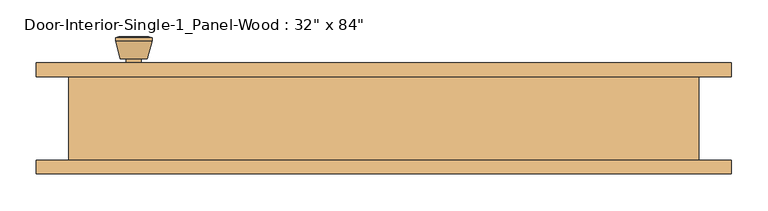
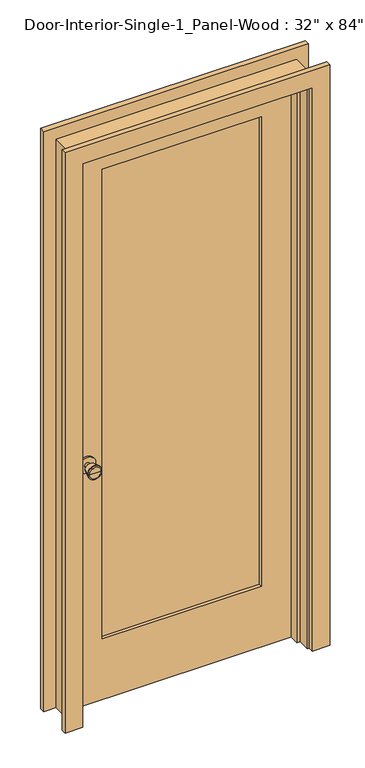
"""IFC4 building model written with IfcOpenShell, lengths in millimetres: door geometry."""

from ifc_helpers import new_model, si_unit, point, frame, frame_2d, origin, place, context, project, spatial, polyline, circle_curve, trimmed, segment, composite_curve, outline, extrude, faceted_brep, source, transform, mapped, element, save
from ifc_brep_helpers import plane_surface, cylinder_surface, revolved_surface, advanced_brep


def door_643e272e(model_context):
    return source(origin(), model_context, "Body", "SolidModel", [
        advanced_brep(
        [(-342.9, 13.05, 914.4), (-332.9, 13.05, 914.4), (-352.9, 13.05, 914.4), (-322.4241324, -35.95, 914.4), (-342.9, -35.95, 914.4), (-363.3758676, -35.95, 914.4), (-317.9, -34.1221319, 914.4), (-367.9, -34.1221319, 914.4), (-317.9, -30.6584537, 914.4), (-367.9, -30.6584537, 914.4), (-324.263764, -5.95, 914.4), (-361.536236, -5.95, 914.4), (-332.9, -5.95, 914.4), (-352.9, -5.95, 914.4)],
        [
            (0, 1),
            (1, 2, circle_curve(frame((-342.9, 13.05, 914.4), z_axis=(0.0, 1.0, 0.0), x_axis=(-1.0, 0.0, 0.0)), 10.0)),
            (2, 0),
            (2, 1, circle_curve(frame((-342.9, 13.05, 914.4), z_axis=(0.0, 1.0, 0.0), x_axis=(-1.0, 0.0, 0.0)), 10.0)),
            (3, 4),
            (4, 5),
            (5, 3, circle_curve(frame((-342.9, -35.95, 914.4), z_axis=(0.0, -1.0, 0.0), x_axis=(-1.0, 0.0, 0.0)), 20.4758676)),
            (3, 5, circle_curve(frame((-342.9, -35.95, 914.4), z_axis=(0.0, -1.0, 0.0), x_axis=(-1.0, 0.0, 0.0)), 20.4758676)),
            (6, 3),
            (5, 7),
            (7, 6, circle_curve(frame((-342.9, -34.1221319, 914.4), z_axis=(0.0, -1.0, 0.0), x_axis=(-1.0, 0.0, 0.0)), 25.0)),
            (6, 7, circle_curve(frame((-342.9, -34.1221319, 914.4), z_axis=(0.0, -1.0, 0.0), x_axis=(-1.0, 0.0, 0.0)), 25.0)),
            (8, 6),
            (7, 9),
            (9, 8, circle_curve(frame((-342.9, -30.6584537, 914.4), z_axis=(0.0, -1.0, 0.0), x_axis=(-1.0, 0.0, 0.0)), 25.0)),
            (8, 9, circle_curve(frame((-342.9, -30.6584537, 914.4), z_axis=(0.0, -1.0, 0.0), x_axis=(-1.0, 0.0, 0.0)), 25.0)),
            (10, 8),
            (9, 11),
            (11, 10, circle_curve(frame((-342.9, -5.95, 914.4), z_axis=(0.0, -1.0, 0.0), x_axis=(-1.0, 0.0, 0.0)), 18.636236)),
            (10, 11, circle_curve(frame((-342.9, -5.95, 914.4), z_axis=(0.0, -1.0, 0.0), x_axis=(-1.0, 0.0, 0.0)), 18.636236)),
            (12, 10),
            (11, 13),
            (13, 12, circle_curve(frame((-342.9, -5.95, 914.4), z_axis=(0.0, -1.0, 0.0), x_axis=(-1.0, 0.0, 0.0)), 10.0)),
            (12, 13, circle_curve(frame((-342.9, -5.95, 914.4), z_axis=(0.0, -1.0, 0.0), x_axis=(-1.0, 0.0, 0.0)), 10.0)),
            (1, 12),
            (13, 2),
        ],
        [
            plane_surface(frame((-342.9, 13.05, 914.4), z_axis=(0.0, 1.0, 0.0), x_axis=(-1.0, 0.0, 0.0))),
            plane_surface(frame((-342.9, -35.95, 914.4), z_axis=(0.0, -1.0, 0.0), x_axis=(-1.0, 0.0, 0.0))),
            revolved_surface(polyline([(-363.3758676, -35.95, 914.4), (-367.9, -34.1221319, 914.4)]), (-342.9, 13.05, 914.4), (0.0, 1.0, 0.0)),
            cylinder_surface(frame((-342.9, 13.05, 914.4), z_axis=(0.0, 1.0, 0.0), x_axis=(-1.0, 0.0, 0.0)), 25.0),
            revolved_surface(polyline([(-367.9, -30.6584537, 914.4), (-361.536236, -5.95, 914.4)]), (-342.9, 13.05, 914.4), (0.0, 1.0, 0.0)),
            plane_surface(frame((-342.9, -5.95, 914.4), z_axis=(0.0, 1.0, 0.0), x_axis=(-1.0, 0.0, 0.0))),
            cylinder_surface(frame((-342.9, 13.05, 914.4), z_axis=(0.0, 1.0, 0.0), x_axis=(-1.0, 0.0, 0.0)), 10.0),
        ],
        [
            (0, [[1, 2, 3]]),
            (0, [[-3, 4, -1]]),
            (1, [[5, 6, 7]]),
            (1, [[-6, -5, 8]]),
            (2, [[9, -7, 10, 11]]),
            (2, [[-10, -8, -9, 12]]),
            (3, [[13, -11, 14, 15]]),
            (3, [[-14, -12, -13, 16]]),
            (4, [[17, -15, 18, 19]]),
            (4, [[-18, -16, -17, 20]]),
            (5, [[21, -19, 22, 23]]),
            (5, [[-22, -20, -21, 24]]),
            (6, [[25, -23, 26, -2]]),
            (6, [[-26, -24, -25, -4]]),
        ],
    ),
        extrude(outline(composite_curve([segment(trimmed(circle_curve(frame_2d((914.4, -342.9)), 30.0), [point((914.4, -372.9))], [point((914.4, -312.9))], False, "CARTESIAN"), True, "CONTINUOUS"), segment(trimmed(circle_curve(frame_2d((914.4, -342.9)), 30.0), [point((914.4, -312.9))], [point((914.4, -372.9))], False, "CARTESIAN"), True, "CONTINUOUS")], self_intersect=False)), frame((0.0, 13.05, 0.0), z_axis=(0.0, 1.0, 0.0), x_axis=(0.0, 0.0, 1.0)), (0.0, 0.0, 1.0), 6.0),
        advanced_brep(
        [(-342.9, 59.975, 914.4), (-352.9, 59.975, 914.4), (-332.9, 59.975, 914.4), (-322.4241324, 108.975, 914.4), (-363.3758676, 108.975, 914.4), (-342.9, 108.975, 914.4), (-317.9, 107.1471319, 914.4), (-367.9, 107.1471319, 914.4), (-317.9, 103.6834537, 914.4), (-367.9, 103.6834537, 914.4), (-324.263764, 78.975, 914.4), (-361.536236, 78.975, 914.4), (-332.9, 78.975, 914.4), (-352.9, 78.975, 914.4)],
        [
            (0, 1),
            (1, 2, circle_curve(frame((-342.9, 59.975, 914.4), z_axis=(0.0, -1.0, 0.0), x_axis=(-1.0, 0.0, 0.0)), 10.0)),
            (2, 0),
            (2, 1, circle_curve(frame((-342.9, 59.975, 914.4), z_axis=(0.0, -1.0, 0.0), x_axis=(-1.0, 0.0, 0.0)), 10.0)),
            (3, 4, circle_curve(frame((-342.9, 108.975, 914.4), z_axis=(0.0, 1.0, 0.0), x_axis=(-1.0, 0.0, 0.0)), 20.4758676)),
            (4, 5),
            (5, 3),
            (4, 3, circle_curve(frame((-342.9, 108.975, 914.4), z_axis=(0.0, 1.0, 0.0), x_axis=(-1.0, 0.0, 0.0)), 20.4758676)),
            (6, 7, circle_curve(frame((-342.9, 107.1471319, 914.4), z_axis=(0.0, 1.0, 0.0), x_axis=(-1.0, 0.0, 0.0)), 25.0)),
            (7, 4),
            (3, 6),
            (7, 6, circle_curve(frame((-342.9, 107.1471319, 914.4), z_axis=(0.0, 1.0, 0.0), x_axis=(-1.0, 0.0, 0.0)), 25.0)),
            (8, 9, circle_curve(frame((-342.9, 103.6834537, 914.4), z_axis=(0.0, 1.0, 0.0), x_axis=(-1.0, 0.0, 0.0)), 25.0)),
            (9, 7),
            (6, 8),
            (9, 8, circle_curve(frame((-342.9, 103.6834537, 914.4), z_axis=(0.0, 1.0, 0.0), x_axis=(-1.0, 0.0, 0.0)), 25.0)),
            (10, 11, circle_curve(frame((-342.9, 78.975, 914.4), z_axis=(0.0, 1.0, 0.0), x_axis=(-1.0, 0.0, 0.0)), 18.636236)),
            (11, 9),
            (8, 10),
            (11, 10, circle_curve(frame((-342.9, 78.975, 914.4), z_axis=(0.0, 1.0, 0.0), x_axis=(-1.0, 0.0, 0.0)), 18.636236)),
            (12, 13, circle_curve(frame((-342.9, 78.975, 914.4), z_axis=(0.0, 1.0, 0.0), x_axis=(-1.0, 0.0, 0.0)), 10.0)),
            (13, 11),
            (10, 12),
            (13, 12, circle_curve(frame((-342.9, 78.975, 914.4), z_axis=(0.0, 1.0, 0.0), x_axis=(-1.0, 0.0, 0.0)), 10.0)),
            (1, 13),
            (12, 2),
        ],
        [
            plane_surface(frame((-342.9, 59.975, 914.4), z_axis=(0.0, -1.0, 0.0), x_axis=(-1.0, 0.0, 0.0))),
            plane_surface(frame((-342.9, 108.975, 914.4), z_axis=(0.0, 1.0, 0.0), x_axis=(-1.0, 0.0, 0.0))),
            revolved_surface(polyline([(-363.3758676, 108.975, 914.4), (-367.9, 107.1471319, 914.4)]), (-342.9, 59.975, 914.4), (0.0, -1.0, 0.0)),
            cylinder_surface(frame((-342.9, 59.975, 914.4), z_axis=(0.0, -1.0, 0.0), x_axis=(-1.0, 0.0, 0.0)), 25.0),
            revolved_surface(polyline([(-367.9, 103.6834537, 914.4), (-361.536236, 78.975, 914.4)]), (-342.9, 59.975, 914.4), (0.0, -1.0, 0.0)),
            plane_surface(frame((-342.9, 78.975, 914.4), z_axis=(0.0, -1.0, 0.0), x_axis=(-1.0, 0.0, 0.0))),
            cylinder_surface(frame((-342.9, 59.975, 914.4), z_axis=(0.0, -1.0, 0.0), x_axis=(-1.0, 0.0, 0.0)), 10.0),
        ],
        [
            (0, [[1, 2, 3]]),
            (0, [[-3, 4, -1]]),
            (1, [[5, 6, 7]]),
            (1, [[8, -7, -6]]),
            (2, [[9, 10, -5, 11]]),
            (2, [[12, -11, -8, -10]]),
            (3, [[13, 14, -9, 15]]),
            (3, [[16, -15, -12, -14]]),
            (4, [[17, 18, -13, 19]]),
            (4, [[20, -19, -16, -18]]),
            (5, [[21, 22, -17, 23]]),
            (5, [[24, -23, -20, -22]]),
            (6, [[-2, 25, -21, 26]]),
            (6, [[-4, -26, -24, -25]]),
        ],
    ),
        extrude(outline(composite_curve([segment(trimmed(circle_curve(frame_2d((914.4, -342.9)), 30.0), [point((914.4, -372.9))], [point((914.4, -312.9))], False, "CARTESIAN"), True, "CONTINUOUS"), segment(trimmed(circle_curve(frame_2d((914.4, -342.9)), 30.0), [point((914.4, -312.9))], [point((914.4, -372.9))], False, "CARTESIAN"), True, "CONTINUOUS")], self_intersect=False)), frame((0.0, 53.975, 0.0), z_axis=(0.0, 1.0, 0.0), x_axis=(0.0, 0.0, 1.0)), (0.0, 0.0, 1.0), 6.0),
        faceted_brep([(431.8, 53.975, 0.0), (431.8, -60.325, 0.0), (406.4, -60.325, 0.0), (406.4, -15.875, 0.0), (393.7, -15.875, 0.0), (393.7, 19.05, 0.0), (406.4, 19.05, 0.0), (406.4, 53.975, 0.0), (431.8, 53.975, 2159.0), (431.8, -60.325, 2159.0), (-431.8, -60.325, 2159.0), (-431.8, -60.325, 0.0), (-406.4, -60.325, 0.0), (-406.4, -60.325, 2133.6), (406.4, -60.325, 2133.6), (406.4, -15.875, 2133.6), (-406.4, -15.875, 2133.6), (-406.4, -15.875, 0.0), (-393.7, -15.875, 0.0), (-393.7, -15.875, 2120.9), (393.7, -15.875, 2120.9), (393.7, 19.05, 2120.9), (-393.7, 19.05, 2120.9), (-393.7, 19.05, 0.0), (-406.4, 19.05, 0.0), (-406.4, 19.05, 2133.6), (406.4, 19.05, 2133.6), (406.4, 53.975, 2133.6), (-406.4, 53.975, 2133.6), (-406.4, 53.975, 0.0), (-431.8, 53.975, 0.0), (-431.8, 53.975, 2159.0)], [[[0, 1, 2, 3, 4, 5, 6, 7]], [[1, 0, 8, 9]], [[2, 1, 9, 10, 11, 12, 13, 14]], [[3, 2, 14, 15]], [[4, 3, 15, 16, 17, 18, 19, 20]], [[5, 4, 20, 21]], [[6, 5, 21, 22, 23, 24, 25, 26]], [[7, 6, 26, 27]], [[0, 7, 27, 28, 29, 30, 31, 8]], [[9, 8, 31, 10]], [[15, 14, 13, 16]], [[21, 20, 19, 22]], [[27, 26, 25, 28]], [[30, 29, 24, 23, 18, 17, 12, 11]], [[10, 31, 30, 11]], [[16, 13, 12, 17]], [[22, 19, 18, 23]], [[28, 25, 24, 29]]]),
        extrude(outline(polyline([(2133.6, -406.4), (0.0, -406.4), (0.0, 406.4), (2133.6, 406.4), (2133.6, -406.4)]), holes=[polyline([(2014.5375, -285.75), (2014.5375, 285.75), (231.775, 285.75), (231.775, -285.75), (2014.5375, -285.75)])]), frame((0.0, 19.05, 0.0), z_axis=(0.0, 1.0, 0.0), x_axis=(0.0, 0.0, 1.0)), (0.0, 0.0, 1.0), 34.925),
        extrude(outline(polyline([(285.75, 30.6916667), (-285.75, 30.6916667), (-285.75, 42.3333333), (285.75, 42.3333333), (285.75, 30.6916667)])), frame((0.0, 0.0, 231.775), z_axis=(0.0, 0.0, 1.0), x_axis=(1.0, 0.0, 0.0)), (0.0, 0.0, 1.0), 1782.7625),
        extrude(outline(polyline([(0.0, 412.75), (0.0, 476.25), (2203.45, 476.25), (2203.45, -476.25), (0.0, -476.25), (0.0, -412.75), (2139.95, -412.75), (2139.95, 412.75), (0.0, 412.75)])), frame((0.0, 53.975, 0.0), z_axis=(0.0, 1.0, 0.0), x_axis=(0.0, 0.0, 1.0)), (0.0, 0.0, 1.0), 19.05),
        extrude(outline(polyline([(0.0, 412.75), (0.0, 476.25), (2203.45, 476.25), (2203.45, -476.25), (0.0, -476.25), (0.0, -412.75), (2139.95, -412.75), (2139.95, 412.75), (0.0, 412.75)])), frame((0.0, -79.375, 0.0), z_axis=(0.0, 1.0, 0.0), x_axis=(0.0, 0.0, 1.0)), (0.0, 0.0, 1.0), 19.05),
    ])


if __name__ == "__main__":
    model = new_model("IFC4")
    model_context = context("Model", 3, world=origin())
    ifc_project = project(units=[si_unit("LENGTHUNIT", "METRE", prefix="MILLI")], contexts=[model_context])
    site = spatial("IfcSite", under=ifc_project)
    building = spatial("IfcBuilding", under=site)
    placement = place(None, origin())
    door_shape = door_643e272e(model_context)
    element("IfcDoor", 1, ObjectType="Door-Interior-Single-1_Panel-Wood : 32\" x 84\"", at=placement, inside=building, context=model_context, shape_type="MappedRepresentation", body=[
        mapped(door_shape, transform((0.0, 0.0, 0.0), x_axis=(1.0, 0.0, 0.0), y_axis=(0.0, 1.0, 0.0), z_axis=(0.0, 0.0, 1.0))),
    ])
    save(model, "model.ifc")

# Revit data of these elements
# Type "Door-Interior-Single-1_Panel-Wood : 32\" x 84\""
#   Type Mark = "8"
#   Assembly Code = "C1020300"
#   Analytic Construction = "Wooden"
#   Top Rail = 0.390625 ft
#   Thickness = 0.114583 ft
#   Thermal Resistance (R) = 2.5876 (h·ft²·°F)/BTU
#   Swing Angle [instance default] = 90.00°
#   Stiles = 0.395833 ft
#   Rough Width = 2.833333 ft
#   Rough Height = 7.083333 ft
#   Height = 7 ft
#   Width = 2.666667 ft
#   Heat Transfer Coefficient (U) = 0.3865 BTU/(h·ft²·°F)
#   Bottom Rail = 0.760417 ft
#   Trim Material = Cherry
#   Panel Material = Cherry
#   Frame Material = Cherry
#   Door Handle Material = Aluminum
#   Visual Light Transmittance = 0
#   Solar Heat Gain Coefficient = 0
#   Wall Closure = (empty or 0)
#   Function = (empty or 0)
# Element 1 (IfcDoor, "Door-Interior-Single-1_Panel-Wood : 32\" x 84\"")
#   Materials on its faces: "Cherry", "Aluminum"
# Materials
#   "Cherry": class "Wood", colour RGB 226 177 128, transparency 0, Description = "Prunus Serotina", Cost = 0
#   "Aluminum": class "Metal", colour RGB 247 247 247, transparency 0, Description = "Aluminum 6061", Cost = 0
